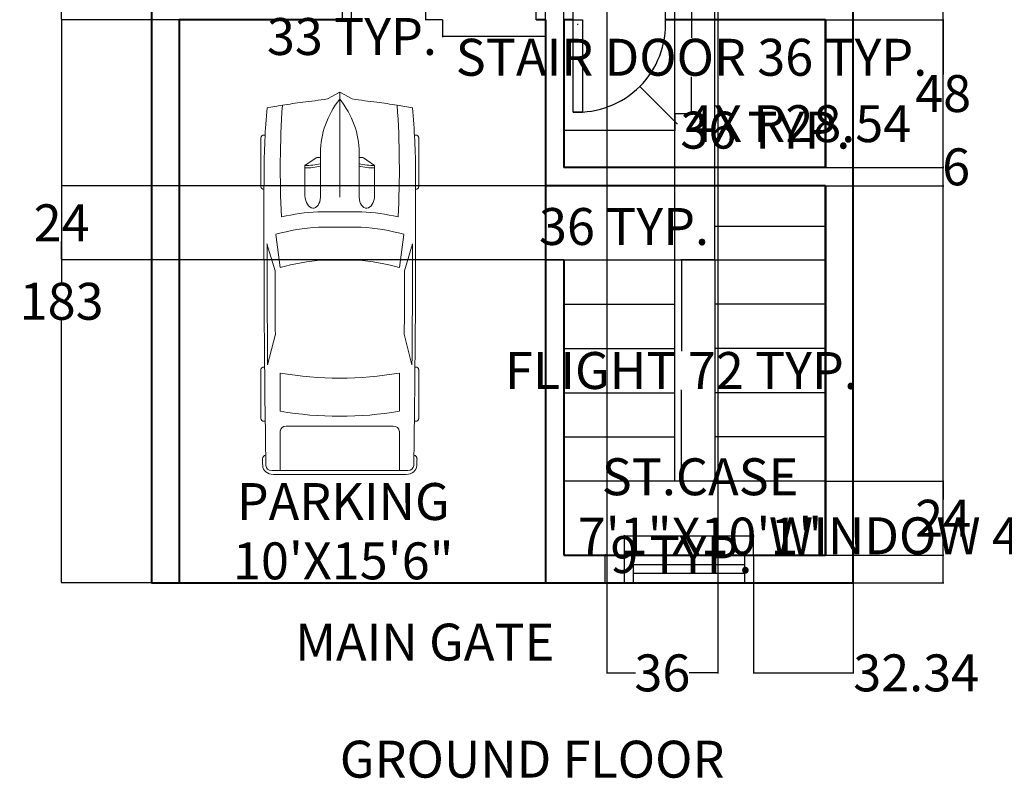
# Model space of a CAD drawing. Units: inches. Extents: x -124 to 612, y -69 to 524.
# Tile 1 of 9: x -33 to 287, y -56 to 190. Entities that reach past the tile are written whole.
import ezdxf
from ezdxf.enums import TextEntityAlignment as Align

# ---------------------------------------------------------------- set-up
doc = ezdxf.new("R2010")
doc.units = ezdxf.units.IN
doc.header["$MEASUREMENT"] = 0
doc.layers.add('5', color=5, linetype='Continuous')
for name, color, linetype, lineweight in [('A-ANNO-DIMS', 2, 'Continuous', 18), ('A-ANNO-TEXT', 1, 'Continuous', 18), ('A-AREA-IDEN', 1, 'Continuous', 18), ('A-DOOR', 4, 'Continuous', 25), ('A-FLOR-STRS', 2, 'Continuous', 25), ('A-GLAZ', 5, 'Continuous', 18), ('A-SITE-VEHI', 8, 'Continuous', 13), ('A-WALL', 7, 'Continuous', 40)]:
    doc.layers.add(name, color=color, linetype=linetype, lineweight=lineweight)
doc.styles.get("Standard").update_dxf_attribs({"font": 'arial.ttf'})
doc.dimstyles.get("Standard").update_dxf_attribs({"dimtxt": 12, "dimasz": 0.18, "dimexe": 0.18, "dimexo": 0.0625, "dimgap": 0.09, "dimtad": 0, "dimtih": 1, "dimtoh": 1, "dimdec": 0, "dimzin": 0, "dimdsep": 46, "dimlunit": 4, "dimtxsty": 'Standard', "dimcen": 0.09, "dimadec": 0, "dimazin": 0, "dimtfac": 1, "dimtdec": 0, "dimtofl": 0, "dimtmove": 0, "dimatfit": 3, "dimfxl": 1, "dimtolj": 1, "dimtzin": 0, "dimarcsym": 0})

# ---------------------------------------------------------------- blocks, each defined once
blk = doc.blocks.new('*U10')
for p, q in [((1182, 988), (568, 988)), ((3472, 988), (4087, 988)), ((536, 950), (536, 936)), ((1214, 950), (1214, 950)), ((2235, 810), (1899, 912)), ((3412, 904), (3030, 807)), ((3440, 942), (3440, 950)), ((4119, 950), (4119, 934)), ((1779, 801), (2195, 746)), ((3516, 746), (3994, 746)), ((4736, 746), (4242, 746)), ((4736, -851), (4736, 851)), ((4785, -832), (4785, 832)), ((4179, 670), (4179, -670)), ((820, 295), (918, 436)), ((918, 436), (1294, 436)), ((816, 241), (816, 283)), ((1496, -274), (1496, 274)), ((1690, -267), (1690, 267)), ((4736, -267), (4736, 267)), ((83, 156), (3, 10)), ((756, 241), (1313, 241)), ((2102, 216), (2102, -216)), ((0, 0), (1313, 0)), ((3, -10), (83, -156)), ((756, -241), (1313, -241)), ((816, -241), (816, -283)), ((820, -295), (918, -436)), ((918, -436), (1294, -436)), ((2195, -746), (1779, -801)), ((2235, -810), (1899, -912)), ((3412, -904), (3030, -807)), ((3994, -746), (3516, -746)), ((4242, -746), (4736, -746)), ((536, -950), (536, -936)), ((1214, -950), (1214, -950)), ((3440, -942), (3440, -950)), ((4119, -950), (4119, -934)), ((1182, -988), (568, -988)), ((3472, -988), (4087, -988))]:
    blk.add_line(p, q)
for centre, major_axis, ratio, start_param, end_param in [((568, 950), (0, -37.6), 0.842304, 3.141593, 4.712389), ((1182, 950), (0, 37.6), 0.842304, -1.570796, 0), ((3472, 950), (0, -37.6), 0.842304, 3.141593, 4.712389), ((4087, 950), (0, 37.6), 0.842304, -1.570796, 0), ((6757, -699), (0, 7958), 0.842304, 1.367076, 1.39176), ((1046, -12468), (0, 13417), 0.842304, 0.00281, 0.075598), ((1638, -268113), (0, 269063), 0.842304, -0.013397, 0.002797), ((1638, -268113), (0, -269025), 0.842304, 3.133765, 3.140441), ((4588, 910), (0, 56.4), 0.842304, -0.013017, 1.249894), ((1638, -268131), (0, 269121), 0.842304, -0.013397, -0.013017), ((4673, 851), (0, -75.2), 0.842304, 1.570796, 3.128196), ((4673, 832), (0, -133), 0.842304, 1.570796, 3.128196), ((952, -15087), (0, -15833), 0.842304, 3.096046, 3.200911), ((3436, 137), (0, 2077), 0.842304, 1.245306, 1.50788), ((3800, 71), (0, -2021), 0.842304, 4.372215, 4.640744), ((2433, -93125), (0, -93935), 0.842304, 3.134049, 3.144098), ((434, 0), (0, 3734), 0.842304, 4.511394, 4.913384), ((912, 0), (0, 3734), 0.842304, 4.511394, 4.913384), ((4242, 670), (0, 75.2), 0.842304, 0, 1.570796), ((6583, -699), (0, -7755), 0.842304, 4.528606, 4.561838), ((3414, 137), (0, -2280), 0.842304, 4.449482, 4.652344), ((-5194, 1331), (0, -6374), 0.842304, 1.385369, 1.434372), ((331, 432), (0, 696), 0.842304, 4.435146, 4.718221), ((361, 432), (0, 696), 0.842304, 4.435146, 4.718221), ((1290, 339), (161, -9), 0.603834, -1.395552, 1.581315), ((832, 283), (0, 18.8), 0.842304, 0.879714, 1.570796), ((756, -1185), (0, 1427), 0.842304, 0, 0.590319), ((16, 0), (0, -18.8), 0.842304, 4.131459, 5.293319), ((756, 1185), (0, 1427), 0.842304, 2.551274, 3.141593), ((-5194, -1331), (0, 6374), 0.842304, -1.434372, -1.385369), ((331, -432), (0, -696), 0.842304, 1.564964, 1.848039), ((361, -432), (0, -696), 0.842304, 1.564964, 1.848039), ((3800, -71), (0, -2021), 0.842304, -1.499151, -1.230623), ((832, -283), (0, -18.8), 0.842304, 4.712389, 5.403472), ((3414, -137), (0, -2280), 0.842304, -1.510751, -1.307889), ((3436, -137), (0, -2077), 0.842304, -1.50788, -1.245306), ((6583, 699), (0, 7755), 0.842304, 1.721348, 1.754579), ((6757, 699), (0, 7958), 0.842304, 1.749832, 1.774517), ((952, 15087), (0, -15833), 0.842304, -0.059319, 0.045547), ((4242, -670), (0, -75.2), 0.842304, 4.712389, 6.283185), ((2433, 93125), (0, -93935), 0.842304, -0.002505, 0.007544), ((4673, -851), (0, 75.2), 0.842304, 3.15499, 4.712389), ((4673, -832), (0, -133), 0.842304, 0.013397, 1.570796), ((1046, 12468), (0, -13417), 0.842304, -0.075598, -0.00281), ((568, -950), (0, 37.6), 0.842304, 1.570796, 3.141593), ((1638, 268113), (0, 269063), 0.842304, 3.138796, 3.15499), ((1182, -950), (0, -37.6), 0.842304, 0, 1.570796), ((1638, 268113), (0, -269025), 0.842304, 0.001152, 0.007828), ((3472, -950), (0, -37.6), 0.842304, -1.570796, 0), ((4087, -950), (0, 37.6), 0.842304, 3.141593, 4.712389), ((4588, -910), (0, -56.4), 0.842304, -1.249894, 0.013017), ((1638, 268131), (0, 269121), 0.842304, 3.15461, 3.15499)]:
    blk.add_ellipse(centre, major_axis=major_axis, ratio=ratio, start_param=start_param, end_param=end_param)
at = {"extrusion": (0, 0, -1)}
blk.add_ellipse((1290, -339), major_axis=(161, 9), ratio=0.603834, start_param=-1.395552, end_param=1.581315, dxfattribs=at)
blk = doc.blocks.new('V')
at = {"layer": '5'}
for p, q in [((0, 0), (0, 9)), ((3, 9), (39, 9)), ((3, 0), (3, 9)), ((39, 9), (39, 0)), ((42, 9), (42, 0)), ((3, 6), (39, 6)), ((39, 3), (3, 3)), ((39, 0), (3, 0))]:
    blk.add_line(p, q, dxfattribs=at)
blk = doc.blocks.new('DOOR-30IN-STAIR')
for p, q in [((0, 30.04), (0, 36.04)), ((3, 30.04), (3, 36.04)), ((33, 30.04), (33, 36.04)), ((36, 30.04), (36, 36.04))]:
    blk.add_line(p, q)
blk.add_lwpolyline([(3, 30.04), (6, 30.04), (6, 0.04), (3, 0.04)], close=True)
blk.add_arc((4.5, 28.54), 28.54, 266.9872, 3.0128)
blk = doc.blocks.new('DOOR-30IN-ENTRY-LEAF')
for p, q in [((0, 0), (0, 6)), ((3, 0), (3, 6))]:
    blk.add_line(p, q)
blk.add_lwpolyline([(3, 6), (6, 6), (6, 36), (3, 36)], close=True)
blk.add_arc((4.5, 7.5), 28.54, 356.9872, 93.0128)
blk = doc.blocks.new('STAIR-FLIGHT-36IN')
for p, q in [((36, 0), (36, 72)), ((0, 57.6), (36, 57.6)), ((0, 43.2), (36, 43.2)), ((0, 28.8), (36, 28.8)), ((0, 14.4), (36, 14.4))]:
    blk.add_line(p, q)
blk = doc.blocks.new('*D19')
at = {"layer": 'A-ANNO-DIMS', "color": 0, "lineweight": -2, "transparency": 16777216}
for p, q in [((193.29, 112.03), (182.37, 112.03)), ((182.55, 111.85), (182.55, 82.32)), ((182.55, 40.21), (182.55, 69.73)), ((193.29, 40.03), (182.37, 40.03))]:
    blk.add_line(p, q, dxfattribs=at)
at = {"layer": 'A-ANNO-DIMS', "color": 0, "transparency": 16777216}
for points in [[(182.52, 111.85), (182.58, 111.85), (182.55, 112.03)], [(182.52, 40.21), (182.58, 40.21), (182.55, 40.03)]]:
    blk.add_solid(points, dxfattribs=at)
at = {"layer": 'Defpoints', "color": 0, "transparency": 16777216}
for p in [(193.35, 112.03), (182.55, 40.03), (193.35, 40.03)]:
    blk.add_point(p, dxfattribs=at)
at = {"layer": 'A-ANNO-DIMS', "color": 0, "transparency": 16777216, "insert": (182.55, 76.03), "char_height": 12, "attachment_point": 5}
blk.add_mtext('\\A1;FLIGHT 72 TYP.', dxfattribs=at)
blk = doc.blocks.new('*D20')
at = {"layer": 'A-ANNO-DIMS', "color": 0, "lineweight": -2, "transparency": 16777216}
for p, q in [((193.35, 122.83), (193.17, 122.83)), ((193.35, 112.09), (193.35, 123.01)), ((229.17, 122.83), (193.53, 122.83)), ((229.35, 112.09), (229.35, 123.01))]:
    blk.add_line(p, q, dxfattribs=at)
at = {"layer": 'A-ANNO-DIMS', "color": 0, "transparency": 16777216}
for points in [[(193.53, 122.86), (193.53, 122.8), (193.35, 122.83)], [(229.17, 122.86), (229.17, 122.8), (229.35, 122.83)]]:
    blk.add_solid(points, dxfattribs=at)
at = {"layer": 'Defpoints', "color": 0, "transparency": 16777216}
for p in [(193.35, 122.83), (193.35, 112.03), (229.35, 112.03)]:
    blk.add_point(p, dxfattribs=at)
at = {"layer": 'A-ANNO-DIMS', "color": 0, "transparency": 16777216, "insert": (163.88, 122.83), "char_height": 12, "attachment_point": 5}
blk.add_mtext('\\A1;36 TYP.', dxfattribs=at)
blk = doc.blocks.new('*D35')
at = {"layer": 'A-ANNO-DIMS', "color": 0, "lineweight": -2, "transparency": 16777216}
for p, q in [((164.01, 16.09), (164.01, 22.51)), ((206.01, 16.09), (206.01, 22.51)), ((164.19, 22.33), (205.83, 22.33)), ((206.01, 22.33), (206.19, 22.33))]:
    blk.add_line(p, q, dxfattribs=at)
at = {"layer": 'A-ANNO-DIMS', "color": 0, "transparency": 16777216}
for points in [[(164.19, 22.36), (164.19, 22.3), (164.01, 22.33)], [(205.83, 22.36), (205.83, 22.3), (206.01, 22.33)]]:
    blk.add_solid(points, dxfattribs=at)
at = {"layer": 'Defpoints', "color": 0, "transparency": 16777216}
for p in [(206.01, 22.33), (164.01, 16.03), (206.01, 16.03)]:
    blk.add_point(p, dxfattribs=at)
at = {"layer": 'A-ANNO-DIMS', "color": 0, "transparency": 16777216, "insert": (274.84, 22.33), "char_height": 12, "attachment_point": 5}
blk.add_mtext('\\A1;WINDOW 42 TYP.', dxfattribs=at)
blk = doc.blocks.new('*D36')
at = {"layer": 'A-ANNO-DIMS', "color": 0, "lineweight": -2, "transparency": 16777216}
for p, q in [((163.95, 16.03), (157.53, 16.03)), ((157.71, 16.03), (157.71, 16.21)), ((157.71, 16.21), (157.89, 16.21)), ((157.71, 7.21), (157.71, 15.85)), ((163.95, 7.03), (157.53, 7.03))]:
    blk.add_line(p, q, dxfattribs=at)
at = {"layer": 'A-ANNO-DIMS', "color": 0, "transparency": 16777216}
for points in [[(157.68, 15.85), (157.74, 15.85), (157.71, 16.03)], [(157.68, 7.21), (157.74, 7.21), (157.71, 7.03)]]:
    blk.add_solid(points, dxfattribs=at)
at = {"layer": 'Defpoints', "color": 0, "transparency": 16777216}
for p in [(157.71, 16.03), (164.01, 16.03), (164.01, 7.03)]:
    blk.add_point(p, dxfattribs=at)
at = {"layer": 'A-ANNO-DIMS', "color": 0, "transparency": 16777216, "insert": (182.53, 16.21), "char_height": 12, "attachment_point": 5}
blk.add_mtext('\\A1;9 TYP.', dxfattribs=at)
blk = doc.blocks.new('*D39')
at = {"layer": 'A-ANNO-DIMS', "color": 0, "lineweight": -2, "transparency": 16777216}
for p, q in [((180.41, 196.03), (186, 196.03)), ((185.82, 195.85), (185.82, 184.12)), ((185.82, 159.78), (185.82, 171.51)), ((180.41, 159.6), (186, 159.6))]:
    blk.add_line(p, q, dxfattribs=at)
at = {"layer": 'A-ANNO-DIMS', "color": 0, "transparency": 16777216}
for points in [[(185.79, 195.85), (185.85, 195.85), (185.82, 196.03)], [(185.79, 159.78), (185.85, 159.78), (185.82, 159.6)]]:
    blk.add_solid(points, dxfattribs=at)
at = {"layer": 'Defpoints', "color": 0, "transparency": 16777216}
for p in [(180.35, 196.03), (185.82, 196.03), (180.35, 159.6)]:
    blk.add_point(p, dxfattribs=at)
at = {"layer": 'A-ANNO-DIMS', "color": 0, "transparency": 16777216, "insert": (185.82, 177.82), "char_height": 12, "attachment_point": 5}
blk.add_mtext('\\A1;STAIR DOOR 36 TYP.', dxfattribs=at)
blk = doc.blocks.new('*D40')
at = {"layer": 'A-ANNO-DIMS', "color": 0, "lineweight": -2, "transparency": 16777216}
for p, q in [((144.35, 159.54), (144.35, 153.96)), ((180.35, 159.54), (180.35, 153.96)), ((144.53, 154.14), (180.17, 154.14)), ((180.35, 154.14), (180.53, 154.14))]:
    blk.add_line(p, q, dxfattribs=at)
at = {"layer": 'A-ANNO-DIMS', "color": 0, "transparency": 16777216}
for points in [[(144.53, 154.17), (144.53, 154.11), (144.35, 154.14)], [(180.17, 154.17), (180.17, 154.11), (180.35, 154.14)]]:
    blk.add_solid(points, dxfattribs=at)
at = {"layer": 'Defpoints', "color": 0, "transparency": 16777216}
for p in [(144.35, 159.6), (180.35, 159.6), (180.35, 154.14)]:
    blk.add_point(p, dxfattribs=at)
at = {"layer": 'A-ANNO-DIMS', "color": 0, "transparency": 16777216, "insert": (209.82, 154.14), "char_height": 12, "attachment_point": 5}
blk.add_mtext('\\A1;36 TYP.', dxfattribs=at)
blk = doc.blocks.new('*D41')
at = {"layer": 'A-ANNO-DIMS', "color": 0, "lineweight": -2, "transparency": 16777216}
for p, q in [((104.86, 226.45), (99.28, 226.45)), ((99.46, 226.27), (99.46, 214.46)), ((99.46, 190.21), (99.46, 202.02)), ((104.86, 190.03), (99.28, 190.03))]:
    blk.add_line(p, q, dxfattribs=at)
at = {"layer": 'A-ANNO-DIMS', "color": 0, "transparency": 16777216}
for points in [[(99.43, 226.27), (99.49, 226.27), (99.46, 226.45)], [(99.43, 190.21), (99.49, 190.21), (99.46, 190.03)]]:
    blk.add_solid(points, dxfattribs=at)
at = {"layer": 'Defpoints', "color": 0, "transparency": 16777216}
for p in [(99.46, 226.45), (104.93, 226.45), (104.93, 190.03)]:
    blk.add_point(p, dxfattribs=at)
at = {"layer": 'A-ANNO-DIMS', "color": 0, "transparency": 16777216, "insert": (99.46, 208.24), "char_height": 12, "attachment_point": 5}
blk.add_mtext('\\A1;LEAF 36 TYP.', dxfattribs=at)
blk = doc.blocks.new('*D42')
at = {"layer": 'A-ANNO-DIMS', "color": 0, "lineweight": -2, "transparency": 16777216}
for p, q in [((104.93, 189.97), (104.93, 184.39)), ((138.35, 189.97), (138.35, 184.39)), ((104.93, 184.57), (104.75, 184.57)), ((138.17, 184.57), (105.11, 184.57))]:
    blk.add_line(p, q, dxfattribs=at)
at = {"layer": 'A-ANNO-DIMS', "color": 0, "transparency": 16777216}
for points in [[(105.11, 184.6), (105.11, 184.54), (104.93, 184.57)], [(138.17, 184.6), (138.17, 184.54), (138.35, 184.57)]]:
    blk.add_solid(points, dxfattribs=at)
at = {"layer": 'Defpoints', "color": 0, "transparency": 16777216}
for p in [(104.93, 190.03), (138.35, 190.03), (104.93, 184.57)]:
    blk.add_point(p, dxfattribs=at)
at = {"layer": 'A-ANNO-DIMS', "color": 0, "transparency": 16777216, "insert": (75.45, 184.57), "char_height": 12, "attachment_point": 5}
blk.add_mtext('\\A1;33 TYP.', dxfattribs=at)
blk = doc.blocks.new('*D48')
at = {"layer": 'A-ANNO-DIMS', "color": 0, "lineweight": -2, "transparency": 16777216}
for p, q in [((238.41, 487.03), (267.78, 487.03)), ((267.6, 486.85), (267.6, 253.25)), ((267.6, 7.21), (267.6, 240.81)), ((238.41, 7.03), (267.78, 7.03))]:
    blk.add_line(p, q, dxfattribs=at)
at = {"layer": 'A-ANNO-DIMS', "color": 0, "transparency": 16777216}
for points in [[(267.57, 486.85), (267.63, 486.85), (267.6, 487.03)], [(267.57, 7.21), (267.63, 7.21), (267.6, 7.03)]]:
    blk.add_solid(points, dxfattribs=at)
at = {"layer": 'Defpoints', "color": 0, "transparency": 16777216}
for p in [(238.35, 487.03), (267.6, 487.03), (238.35, 7.03)]:
    blk.add_point(p, dxfattribs=at)
at = {"layer": 'A-ANNO-DIMS', "color": 0, "transparency": 16777216, "insert": (267.6, 247.03), "char_height": 12, "attachment_point": 5}
blk.add_mtext('\\A1;480', dxfattribs=at)
blk = doc.blocks.new('*D52')
at = {"layer": 'A-ANNO-DIMS', "color": 0, "lineweight": -2, "transparency": 16777216}
for p, q in [((158.35, 327.97), (158.35, -22.4)), ((194.35, 327.97), (194.35, -22.4)), ((158.53, -22.22), (167.67, -22.22)), ((194.17, -22.22), (185.03, -22.22))]:
    blk.add_line(p, q, dxfattribs=at)
at = {"layer": 'A-ANNO-DIMS', "color": 0, "transparency": 16777216}
for points in [[(158.53, -22.19), (158.53, -22.25), (158.35, -22.22)], [(194.17, -22.19), (194.17, -22.25), (194.35, -22.22)]]:
    blk.add_solid(points, dxfattribs=at)
at = {"layer": 'Defpoints', "color": 0, "transparency": 16777216}
for p in [(158.35, 328.03), (194.35, 328.03), (194.35, -22.22)]:
    blk.add_point(p, dxfattribs=at)
at = {"layer": 'A-ANNO-DIMS', "color": 0, "transparency": 16777216, "insert": (176.35, -22.22), "char_height": 12, "attachment_point": 5}
blk.add_mtext('\\A1;36', dxfattribs=at)
blk = doc.blocks.new('*D55')
at = {"layer": 'A-ANNO-DIMS', "color": 0, "lineweight": -2, "transparency": 16777216}
for p, q in [((19.29, 190.03), (-19.08, 190.03)), ((-18.9, 189.85), (-18.9, 104.75)), ((-18.9, 7.21), (-18.9, 92.31)), ((10.29, 7.03), (-19.08, 7.03))]:
    blk.add_line(p, q, dxfattribs=at)
at = {"layer": 'A-ANNO-DIMS', "color": 0, "transparency": 16777216}
for points in [[(-18.93, 189.85), (-18.87, 189.85), (-18.9, 190.03)], [(-18.93, 7.21), (-18.87, 7.21), (-18.9, 7.03)]]:
    blk.add_solid(points, dxfattribs=at)
at = {"layer": 'Defpoints', "color": 0, "transparency": 16777216}
for p in [(-18.9, 190.03), (19.35, 190.03), (10.35, 7.03)]:
    blk.add_point(p, dxfattribs=at)
at = {"layer": 'A-ANNO-DIMS', "color": 0, "transparency": 16777216, "insert": (-18.9, 98.53), "char_height": 12, "attachment_point": 5}
blk.add_mtext('\\A1;183', dxfattribs=at)
blk = doc.blocks.new('*D56')
at = {"layer": 'A-ANNO-DIMS', "color": 0, "lineweight": -2, "transparency": 16777216}
for p, q in [((19.29, 328.03), (-19.08, 328.03)), ((-18.9, 327.85), (-18.9, 265.25)), ((-18.9, 190.21), (-18.9, 252.81)), ((19.29, 190.03), (-19.08, 190.03))]:
    blk.add_line(p, q, dxfattribs=at)
at = {"layer": 'A-ANNO-DIMS', "color": 0, "transparency": 16777216}
for points in [[(-18.93, 327.85), (-18.87, 327.85), (-18.9, 328.03)], [(-18.93, 190.21), (-18.87, 190.21), (-18.9, 190.03)]]:
    blk.add_solid(points, dxfattribs=at)
at = {"layer": 'Defpoints', "color": 0, "transparency": 16777216}
for p in [(-18.9, 328.03), (19.35, 328.03), (19.35, 190.03)]:
    blk.add_point(p, dxfattribs=at)
at = {"layer": 'A-ANNO-DIMS', "color": 0, "transparency": 16777216, "insert": (-18.9, 259.03), "char_height": 12, "attachment_point": 5}
blk.add_mtext('\\A1;138', dxfattribs=at)
blk = doc.blocks.new('*D61')
at = {"layer": 'A-ANNO-DIMS', "color": 0, "lineweight": -2, "transparency": 16777216}
for p, q in [((138.29, 136.03), (-19.08, 136.03)), ((-18.9, 135.85), (-18.9, 130.14)), ((-18.9, 112.21), (-18.9, 117.91)), ((144.29, 112.03), (-19.08, 112.03))]:
    blk.add_line(p, q, dxfattribs=at)
at = {"layer": 'A-ANNO-DIMS', "color": 0, "transparency": 16777216}
for points in [[(-18.93, 135.85), (-18.87, 135.85), (-18.9, 136.03)], [(-18.93, 112.21), (-18.87, 112.21), (-18.9, 112.03)]]:
    blk.add_solid(points, dxfattribs=at)
at = {"layer": 'Defpoints', "color": 0, "transparency": 16777216}
for p in [(-18.9, 136.03), (138.35, 136.03), (144.35, 112.03)]:
    blk.add_point(p, dxfattribs=at)
at = {"layer": 'A-ANNO-DIMS', "color": 0, "transparency": 16777216, "insert": (-18.9, 124.03), "char_height": 12, "attachment_point": 5}
blk.add_mtext('\\A1;24', dxfattribs=at)
blk = doc.blocks.new('*D62')
at = {"layer": 'A-ANNO-DIMS', "color": 0, "lineweight": -2, "transparency": 16777216}
for p, q in [((229.41, 40.03), (267.78, 40.03)), ((267.6, 39.85), (267.6, 34.14)), ((267.6, 16.21), (267.6, 21.91)), ((229.41, 16.03), (267.78, 16.03))]:
    blk.add_line(p, q, dxfattribs=at)
at = {"layer": 'A-ANNO-DIMS', "color": 0, "transparency": 16777216}
for points in [[(267.57, 39.85), (267.63, 39.85), (267.6, 40.03)], [(267.57, 16.21), (267.63, 16.21), (267.6, 16.03)]]:
    blk.add_solid(points, dxfattribs=at)
at = {"layer": 'Defpoints', "color": 0, "transparency": 16777216}
for p in [(229.35, 40.03), (267.6, 40.03), (229.35, 16.03)]:
    blk.add_point(p, dxfattribs=at)
at = {"layer": 'A-ANNO-DIMS', "color": 0, "transparency": 16777216, "insert": (267.6, 28.03), "char_height": 12, "attachment_point": 5}
blk.add_mtext('\\A1;24', dxfattribs=at)
blk = doc.blocks.new('*D63')
at = {"layer": 'A-ANNO-DIMS', "color": 0, "lineweight": -2, "transparency": 16777216}
for p, q in [((229.41, 190.03), (267.78, 190.03)), ((267.6, 189.85), (267.6, 172.25)), ((267.6, 142.21), (267.6, 159.81)), ((229.41, 142.03), (267.78, 142.03))]:
    blk.add_line(p, q, dxfattribs=at)
at = {"layer": 'A-ANNO-DIMS', "color": 0, "transparency": 16777216}
for points in [[(267.57, 189.85), (267.63, 189.85), (267.6, 190.03)], [(267.57, 142.21), (267.63, 142.21), (267.6, 142.03)]]:
    blk.add_solid(points, dxfattribs=at)
at = {"layer": 'Defpoints', "color": 0, "transparency": 16777216}
for p in [(229.35, 190.03), (267.6, 190.03), (229.35, 142.03)]:
    blk.add_point(p, dxfattribs=at)
at = {"layer": 'A-ANNO-DIMS', "color": 0, "transparency": 16777216, "insert": (267.6, 166.03), "char_height": 12, "attachment_point": 5}
blk.add_mtext('\\A1;48', dxfattribs=at)
blk = doc.blocks.new('*D64')
at = {"layer": 'A-ANNO-DIMS', "color": 0, "lineweight": -2, "transparency": 16777216}
for p, q in [((206.01, 6.97), (206.01, -22.4)), ((238.35, 6.97), (238.35, -22.4)), ((206.19, -22.22), (238.17, -22.22)), ((238.35, -22.22), (238.53, -22.22))]:
    blk.add_line(p, q, dxfattribs=at)
at = {"layer": 'A-ANNO-DIMS', "color": 0, "transparency": 16777216}
for points in [[(206.19, -22.19), (206.19, -22.25), (206.01, -22.22)], [(238.17, -22.19), (238.17, -22.25), (238.35, -22.22)]]:
    blk.add_solid(points, dxfattribs=at)
at = {"layer": 'Defpoints', "color": 0, "transparency": 16777216}
for p in [(206.01, 7.03), (238.35, 7.03), (238.35, -22.22)]:
    blk.add_point(p, dxfattribs=at)
at = {"layer": 'A-ANNO-DIMS', "color": 0, "transparency": 16777216, "insert": (258.84, -22.22), "char_height": 12, "attachment_point": 5}
blk.add_mtext('\\A1;32.34', dxfattribs=at)
blk = doc.blocks.new('*D65')
at = {"layer": 'A-ANNO-DIMS', "color": 0, "lineweight": -2, "transparency": 16777216}
for p, q in [((180.35, 112.09), (180.35, 516.46)), ((180.53, 516.28), (193.17, 516.28)), ((193.35, 112.09), (193.35, 516.46)), ((193.35, 516.28), (193.53, 516.28))]:
    blk.add_line(p, q, dxfattribs=at)
at = {"layer": 'A-ANNO-DIMS', "color": 0, "transparency": 16777216}
for points in [[(180.53, 516.31), (180.53, 516.25), (180.35, 516.28)], [(193.17, 516.31), (193.17, 516.25), (193.35, 516.28)]]:
    blk.add_solid(points, dxfattribs=at)
at = {"layer": 'Defpoints', "color": 0, "transparency": 16777216}
for p in [(193.35, 516.28), (180.35, 112.03), (193.35, 112.03)]:
    blk.add_point(p, dxfattribs=at)
at = {"layer": 'A-ANNO-DIMS', "color": 0, "transparency": 16777216, "insert": (201.65, 516.28), "char_height": 12, "attachment_point": 5}
blk.add_mtext('\\A1;13', dxfattribs=at)
blk = doc.blocks.new('*D66')
at = {"layer": 'A-ANNO-DIMS', "color": 0, "lineweight": -2, "transparency": 16777216}
for p, q in [((229.41, 142.03), (267.78, 142.03)), ((267.6, 142.03), (267.6, 142.21)), ((267.6, 142.21), (267.78, 142.21)), ((267.6, 136.21), (267.6, 141.85)), ((229.41, 136.03), (267.78, 136.03))]:
    blk.add_line(p, q, dxfattribs=at)
at = {"layer": 'A-ANNO-DIMS', "color": 0, "transparency": 16777216}
for points in [[(267.57, 141.85), (267.63, 141.85), (267.6, 142.03)], [(267.57, 136.21), (267.63, 136.21), (267.6, 136.03)]]:
    blk.add_solid(points, dxfattribs=at)
at = {"layer": 'Defpoints', "color": 0, "transparency": 16777216}
for p in [(229.35, 142.03), (267.6, 142.03), (229.35, 136.03)]:
    blk.add_point(p, dxfattribs=at)
at = {"layer": 'A-ANNO-DIMS', "color": 0, "transparency": 16777216, "insert": (271.83, 142.21), "char_height": 12, "attachment_point": 5}
blk.add_mtext('\\A1;6', dxfattribs=at)
blk = doc.blocks.new('*D72')
at = {"layer": 'A-ANNO-DIMS', "color": 0, "lineweight": -2, "transparency": 16777216}
for p, q in [((148.76, 188.53), (148.94, 188.53)), ((148.85, 188.44), (148.85, 188.62)), ((181.14, 156.24), (169.16, 168.22)), ((181.32, 156.24), (181.14, 156.24))]:
    blk.add_line(p, q, dxfattribs=at)
at = {"layer": 'A-ANNO-DIMS', "color": 0, "transparency": 16777216}
blk.add_solid([(169.18, 168.24), (169.14, 168.2), (169.03, 168.35)], dxfattribs=at)
at = {"layer": 'Defpoints', "color": 0, "transparency": 16777216}
for p in [(148.85, 188.53), (169.03, 168.35)]:
    blk.add_point(p, dxfattribs=at)
at = {"layer": 'A-ANNO-DIMS', "color": 0, "transparency": 16777216, "insert": (220.51, 156.24), "char_height": 12, "attachment_point": 5}
blk.add_mtext('\\A1;4X R28.54', dxfattribs=at)

msp = doc.modelspace()

# ---------------------------------------------------------------- linework, layer by layer
at = {"layer": 'A-FLOR-STRS'}
for p, q in [((144.3513, 136.0291), (229.3513, 136.0291)), ((229.3513, 136.0291), (229.3513, 16.0291)), ((138.3513, 112.0291), (229.3513, 112.0291)), ((144.3513, 16.0291), (144.3513, 112.0291)), ((229.3513, 40.0291), (144.3513, 40.0291)), ((229.3513, 16.0291), (144.3513, 16.0291))]:
    msp.add_line(p, q, dxfattribs=at)
msp.add_lwpolyline([(138.3513, 121.1346, 0, 0, 0), (211.4493, 121.1346, 0, 0, 0), (211.4493, 68.8291, 12, 0, 0), (211.4493, 40.0291, 0, 0, 0)], format="xyseb", dxfattribs=at)
at = {"layer": 'A-WALL'}
for p, q in [((19.3513, 190.0291), (19.3513, 7.0291)), ((75.3513, 190.0291), (19.3513, 190.0291)), ((138.3513, 190.0291), (135.3513, 190.0291)), ((138.3513, 190.0291), (138.3513, 7.0291)), ((144.3513, 190.0291), (144.3513, 142.0291)), ((147.3513, 190.0291), (144.3513, 190.0291)), ((229.3513, 190.0291), (177.3513, 190.0291)), ((229.3513, 190.0291), (229.3513, 142.0291)), ((229.3513, 142.0291), (229.3513, 190.0291)), ((229.3513, 142.0291), (144.3513, 142.0291)), ((229.3513, 136.0291), (138.3513, 136.0291)), ((229.3513, 16.0291), (229.3513, 136.0291)), ((229.3513, 136.0291), (229.3513, 16.0291)), ((144.3513, 112.0291), (144.3513, 16.0291)), ((144.3513, 16.0291), (229.3513, 16.0291))]:
    msp.add_line(p, q, dxfattribs=at)
msp.add_lwpolyline([(10.3513, 7.0291), (238.3513, 7.0291), (238.3513, 487.0291), (10.3513, 487.0291)], close=True, dxfattribs=at)

# ---------------------------------------------------------------- block references
at = {"layer": 'A-DOOR'}
for name, p in [('DOOR-30IN-ENTRY-LEAF', (72.351, 190.029)), ('DOOR-30IN-STAIR', (144.351, 159.99))]:
    msp.add_blockref(name, p, dxfattribs=at)
at = {"layer": 'A-DOOR', "extrusion": (0, 0, -1), "zscale": -1}
msp.add_blockref('DOOR-30IN-ENTRY-LEAF', (-138.3516, 190.029), dxfattribs=at)
at = {"layer": 'A-FLOR-STRS'}
msp.add_blockref('STAIR-FLIGHT-36IN', (144.351, 40.029), dxfattribs=at)
at = {"layer": 'A-FLOR-STRS', "rotation": 180}
msp.add_blockref('STAIR-FLIGHT-36IN', (229.3516, 112.0291), dxfattribs=at)
at = {"layer": 'A-GLAZ'}
msp.add_blockref('V', (164.0117, 7.0291), dxfattribs=at)
at = {"layer": 'A-SITE-VEHI', "xscale": 0.0259494120509158, "yscale": 0.0259494120509158, "zscale": 0.0259494120509158, "rotation": 270}
msp.add_blockref('*U10', (71.5116, 166.4362), dxfattribs=at)

# ---------------------------------------------------------------- texts
at = {"layer": 'A-ANNO-TEXT'}
for s, p in [('MAIN GATE', (99.1026, -18.2167)), ('GROUND FLOOR', (134.0279, -56.2641))]:
    msp.add_text(s, height=12, dxfattribs=at).set_placement(p, align=Align.CENTER)
at = {"layer": 'A-AREA-IDEN'}
for s, p in [('ST.CASE', (188.5958, 35.5089)), ('PARKING', (72.6339, 27.4557)), ('7\'1"X10\'1"', (188.5958, 16.2319)), ('10\'X15\'6"', (72.6339, 8.1787))]:
    msp.add_text(s, height=12, dxfattribs=at).set_placement(p, align=Align.CENTER)

# ---------------------------------------------------------------- dimensions: what is measured, and where the dimension line sits
at = {"layer": 'A-ANNO-DIMS'}
for base, p1, p2, override, picture, middle in [((193.3513, 516.2791), (180.3513, 112.0291), (193.3513, 112.0291), {"dimdec": 0, "dimlfac": 1, "dimrnd": 0, "dimzin": 0, "dimdsep": 46, "dimlunit": 2}, '*D65', (201.6513, 516.2791)), ((194.3513, -22.2209), (158.3513, 328.0291), (194.3513, 328.0291), {"dimdec": 0, "dimlfac": 1, "dimrnd": 0, "dimzin": 0, "dimdsep": 46, "dimlunit": 2}, '*D52', (176.3513, -22.2209)), ((238.3513, -22.2209), (206.0117, 7.0291), (238.3513, 7.0291), {"dimdec": 2, "dimlfac": 1, "dimrnd": 0, "dimzin": 0, "dimdsep": 46, "dimlunit": 2}, '*D64', (258.8396, -22.2209))]:
    dim = msp.add_linear_dim(base=base, p1=p1, p2=p2, dimstyle='Standard', override=override, dxfattribs=at)
    dim.commit()
    dim.dimension.update_dxf_attribs({"geometry": picture, "text_midpoint": middle})
for base, p1, p2, picture, middle in [((267.6013, 487.0291), (238.3513, 7.0291), (238.3513, 487.0291), '*D48', (267.6013, 247.0291)), ((-18.8987, 328.0291), (19.3513, 190.0291), (19.3513, 328.0291), '*D56', (-18.8987, 259.0291)), ((-18.8987, 190.0291), (10.3513, 7.0291), (19.3513, 190.0291), '*D55', (-18.8987, 98.5291)), ((267.6013, 190.0291), (229.3513, 142.0291), (229.3513, 190.0291), '*D63', (267.6013, 166.0291)), ((267.6013, 142.0291), (229.3513, 136.0291), (229.3513, 142.0291), '*D66', (271.8331, 142.2091)), ((-18.8987, 136.0291), (144.3513, 112.0291), (138.3513, 136.0291), '*D61', (-18.8987, 124.0291)), ((267.6013, 40.0291), (229.3513, 16.0291), (229.3513, 40.0291), '*D62', (267.6013, 28.0291))]:
    dim = msp.add_linear_dim(base=base, p1=p1, p2=p2, angle=90, dimstyle='Standard', override={"dimdec": 0, "dimlfac": 1, "dimrnd": 0, "dimzin": 0, "dimdsep": 46, "dimlunit": 2}, dxfattribs=at)
    dim.commit()
    dim.dimension.update_dxf_attribs({"geometry": picture, "text_midpoint": middle})
for base, p1, p2, angle, text, picture, middle in [((99.4623, 226.4543), (104.9261, 190.0291), (104.9261, 226.4543), 90, 'LEAF <> TYP.', '*D41', (99.4623, 208.2417)), ((185.8151, 196.0291), (180.3513, 159.6038), (180.3513, 196.0291), 90, 'STAIR DOOR <> TYP.', '*D39', (185.8151, 177.8164)), ((104.9261, 184.5653), (138.3513, 190.0291), (104.9261, 190.0291), 180, '<> TYP.', '*D42', (75.4542, 184.5653)), ((193.3513, 122.8291), (229.3513, 112.0291), (193.3513, 112.0291), 180, '<> TYP.', '*D20', (163.8794, 122.8291)), ((182.5513, 40.0291), (193.3513, 112.0291), (193.3513, 40.0291), 270, 'FLIGHT <> TYP.', '*D19', (182.5513, 76.0291)), ((157.7117, 16.0291), (164.0117, 7.0291), (164.0117, 16.0291), 90, '<> TYP.', '*D36', (182.526, 16.2091))]:
    dim = msp.add_linear_dim(base=base, p1=p1, p2=p2, angle=angle, text=text, dimstyle='Standard', override={"dimdec": 0, "dimlfac": 1, "dimrnd": 0, "dimzin": 0, "dimdsep": 46, "dimlunit": 2}, dxfattribs=at)
    dim.commit()
    dim.dimension.update_dxf_attribs({"geometry": picture, "text_midpoint": middle})
dim = msp.add_radius_dim(center=(148.8513, 188.5291), mpoint=(169.0316, 168.3484), text='4X <>', dimstyle='Standard', override={"dimdec": 2, "dimlfac": 1, "dimrnd": 0, "dimzin": 0, "dimdsep": 46, "dimlunit": 2}, dxfattribs=at)
dim.commit()
dim.dimension.update_dxf_attribs({"geometry": '*D72', "text_midpoint": (220.5079, 156.2401), "dimtype": 164})
for base, p1, p2, text, picture, middle in [((180.3513, 154.14), (144.3513, 159.6038), (180.3513, 159.6038), '<> TYP.', '*D40', (209.8232, 154.14)), ((206.0117, 22.3291), (164.0117, 16.0291), (206.0117, 16.0291), 'WINDOW <> TYP.', '*D35', (274.8397, 22.3291))]:
    dim = msp.add_linear_dim(base=base, p1=p1, p2=p2, text=text, dimstyle='Standard', override={"dimdec": 0, "dimlfac": 1, "dimrnd": 0, "dimzin": 0, "dimdsep": 46, "dimlunit": 2}, dxfattribs=at)
    dim.commit()
    dim.dimension.update_dxf_attribs({"geometry": picture, "text_midpoint": middle})

doc.saveas('drawing.dxf')
